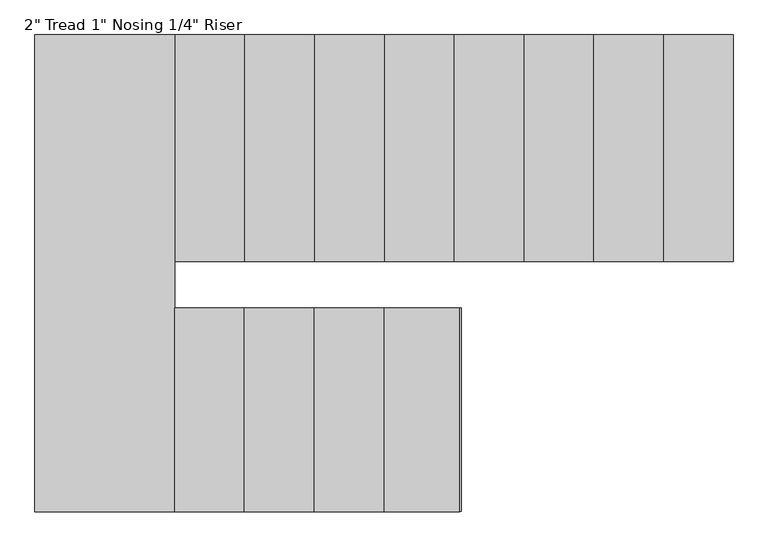
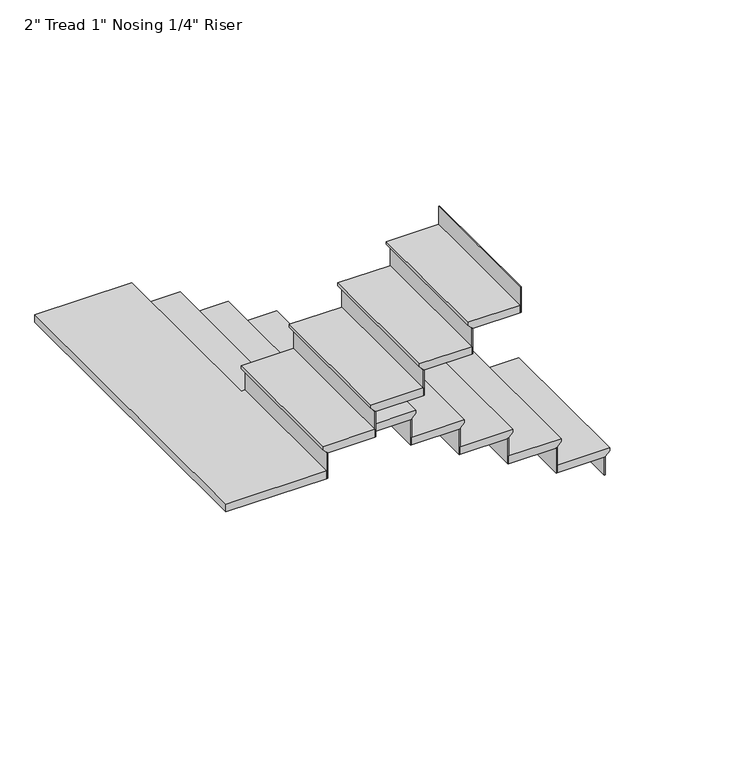
"""IFC4 building model written with IfcOpenShell, lengths in millimetres: stair flight geometry."""

from ifc_helpers import new_model, si_unit, origin, place, context, project, spatial, faceted_brep, source, transform, mapped, element, save


def stair_flight_db34188c(model_context):
    return source(origin(), model_context, "Body", "Brep", [
        faceted_brep([(-569.5630704, 657.3457979, 9599.0833333), (-569.5630704, 657.3457979, 9618.1333333), (-569.5630704, -333.2542021, 9618.1333333), (-569.5630704, -333.2542021, 9599.0833333), (-594.9630704, 657.3457979, 9573.6833333), (-594.9630704, -333.2542021, 9573.6833333), (-899.7630704, 657.3457979, 9618.1333333), (-899.7630704, -333.2542021, 9618.1333333), (-594.9630704, -333.2542021, 9567.3333333), (-899.7630704, -333.2542021, 9567.3333333), (-899.7630704, 657.3457979, 9567.3333333), (-594.9630704, 657.3457979, 9567.3333333)], [[[0, 1, 2, 3]], [[4, 0, 3, 5]], [[2, 1, 6, 7]], [[8, 9, 10, 11]], [[2, 7, 9, 8, 5, 3]], [[8, 11, 4, 5]], [[6, 1, 0, 4, 11, 10]], [[7, 6, 10, 9]]]),
        faceted_brep([(-594.9630704, 657.3457979, 9567.3333333), (-594.9630704, 657.3457979, 9448.8), (-601.3130704, 657.3457979, 9448.8), (-601.3130704, 657.3457979, 9567.3333333), (-594.9630704, -333.2542021, 9567.3333333), (-601.3130704, -333.2542021, 9567.3333333), (-601.3130704, -333.2542021, 9448.8), (-594.9630704, -333.2542021, 9448.8)], [[[0, 1, 2, 3]], [[4, 5, 6, 7]], [[1, 0, 4, 7]], [[2, 1, 7, 6]], [[3, 2, 6, 5]], [[0, 3, 5, 4]]]),
        faceted_brep([(-899.7630704, 657.3457979, 9736.6666667), (-899.7630704, 657.3457979, 9567.3333333), (-906.1130704, 657.3457979, 9567.3333333), (-906.1130704, 657.3457979, 9736.6666667), (-899.7630704, -333.2542021, 9736.6666667), (-906.1130704, -333.2542021, 9736.6666667), (-906.1130704, -333.2542021, 9567.3333333), (-899.7630704, -333.2542021, 9567.3333333)], [[[0, 1, 2, 3]], [[4, 5, 6, 7]], [[1, 0, 4, 7]], [[2, 1, 7, 6]], [[3, 2, 6, 5]], [[0, 3, 5, 4]]]),
        faceted_brep([(-874.3630704, -333.2542021, 9787.4666667), (-874.3630704, 657.3457979, 9787.4666667), (-1204.5630704, 657.3457979, 9787.4666667), (-1204.5630704, -333.2542021, 9787.4666667), (-899.7630704, -333.2542021, 9736.6666667), (-1204.5630704, -333.2542021, 9736.6666667), (-1204.5630704, 657.3457979, 9736.6666667), (-899.7630704, 657.3457979, 9736.6666667), (-899.7630704, -333.2542021, 9743.0166667), (-874.3630704, -333.2542021, 9768.4166667), (-899.7630704, 657.3457979, 9743.0166667), (-874.3630704, 657.3457979, 9768.4166667)], [[[0, 1, 2, 3]], [[4, 5, 6, 7]], [[0, 3, 5, 4, 8, 9]], [[4, 7, 10, 8]], [[2, 1, 11, 10, 7, 6]], [[3, 2, 6, 5]], [[11, 1, 0, 9]], [[10, 11, 9, 8]]]),
        faceted_brep([(-1204.5630704, 657.3457979, 9906.0), (-1204.5630704, 657.3457979, 9736.6666667), (-1210.9130704, 657.3457979, 9736.6666667), (-1210.9130704, 657.3457979, 9906.0), (-1204.5630704, -333.2542021, 9906.0), (-1210.9130704, -333.2542021, 9906.0), (-1210.9130704, -333.2542021, 9736.6666667), (-1204.5630704, -333.2542021, 9736.6666667)], [[[0, 1, 2, 3]], [[4, 5, 6, 7]], [[1, 0, 4, 7]], [[2, 1, 7, 6]], [[3, 2, 6, 5]], [[0, 3, 5, 4]]]),
        faceted_brep([(-1179.1630704, -333.2542021, 9956.8), (-1179.1630704, 657.3457979, 9956.8), (-1509.3630704, 657.3457979, 9956.8), (-1509.3630704, -333.2542021, 9956.8), (-1204.5630704, -333.2542021, 9906.0), (-1509.3630704, -333.2542021, 9906.0), (-1509.3630704, 657.3457979, 9906.0), (-1204.5630704, 657.3457979, 9906.0), (-1204.5630704, -333.2542021, 9912.35), (-1179.1630704, -333.2542021, 9937.75), (-1204.5630704, 657.3457979, 9912.35), (-1179.1630704, 657.3457979, 9937.75)], [[[0, 1, 2, 3]], [[4, 5, 6, 7]], [[0, 3, 5, 4, 8, 9]], [[4, 7, 10, 8]], [[2, 1, 11, 10, 7, 6]], [[3, 2, 6, 5]], [[11, 1, 0, 9]], [[10, 11, 9, 8]]]),
        faceted_brep([(-1509.3630704, 657.3457979, 10075.3333333), (-1509.3630704, 657.3457979, 9906.0), (-1515.7130704, 657.3457979, 9906.0), (-1515.7130704, 657.3457979, 10075.3333333), (-1509.3630704, -333.2542021, 10075.3333333), (-1515.7130704, -333.2542021, 10075.3333333), (-1515.7130704, -333.2542021, 9906.0), (-1509.3630704, -333.2542021, 9906.0)], [[[0, 1, 2, 3]], [[4, 5, 6, 7]], [[1, 0, 4, 7]], [[2, 1, 7, 6]], [[3, 2, 6, 5]], [[0, 3, 5, 4]]]),
        faceted_brep([(-1483.9630704, -333.2542021, 10126.1333333), (-1483.9630704, 657.3457979, 10126.1333333), (-1814.1630704, 657.3457979, 10126.1333333), (-1814.1630704, -333.2542021, 10126.1333333), (-1509.3630704, -333.2542021, 10075.3333333), (-1814.1630704, -333.2542021, 10075.3333333), (-1814.1630704, 657.3457979, 10075.3333333), (-1509.3630704, 657.3457979, 10075.3333333), (-1509.3630704, -333.2542021, 10081.6833333), (-1483.9630704, -333.2542021, 10107.0833333), (-1509.3630704, 657.3457979, 10081.6833333), (-1483.9630704, 657.3457979, 10107.0833333)], [[[0, 1, 2, 3]], [[4, 5, 6, 7]], [[0, 3, 5, 4, 8, 9]], [[4, 7, 10, 8]], [[2, 1, 11, 10, 7, 6]], [[3, 2, 6, 5]], [[11, 1, 0, 9]], [[10, 11, 9, 8]]]),
        faceted_brep([(-1814.1630704, 657.3457979, 10244.6666667), (-1814.1630704, 657.3457979, 10075.3333333), (-1820.5130704, 657.3457979, 10075.3333333), (-1820.5130704, 657.3457979, 10244.6666667), (-1814.1630704, -333.2542021, 10244.6666667), (-1820.5130704, -333.2542021, 10244.6666667), (-1820.5130704, -333.2542021, 10075.3333333), (-1814.1630704, -333.2542021, 10075.3333333)], [[[0, 1, 2, 3]], [[4, 5, 6, 7]], [[1, 0, 4, 7]], [[2, 1, 7, 6]], [[3, 2, 6, 5]], [[0, 3, 5, 4]]]),
        faceted_brep([(-1788.7630704, -333.2542021, 10295.4666667), (-1788.7630704, 657.3457979, 10295.4666667), (-2118.9630704, 657.3457979, 10295.4666667), (-2118.9630704, -333.2542021, 10295.4666667), (-1814.1630704, -333.2542021, 10244.6666667), (-2118.9630704, -333.2542021, 10244.6666667), (-2118.9630704, 657.3457979, 10244.6666667), (-1814.1630704, 657.3457979, 10244.6666667), (-1814.1630704, -333.2542021, 10251.0166667), (-1788.7630704, -333.2542021, 10276.4166667), (-1814.1630704, 657.3457979, 10251.0166667), (-1788.7630704, 657.3457979, 10276.4166667)], [[[0, 1, 2, 3]], [[4, 5, 6, 7]], [[0, 3, 5, 4, 8, 9]], [[4, 7, 10, 8]], [[2, 1, 11, 10, 7, 6]], [[3, 2, 6, 5]], [[11, 1, 0, 9]], [[10, 11, 9, 8]]]),
        faceted_brep([(-2118.9630704, 657.3457979, 10414.0), (-2118.9630704, 657.3457979, 10244.6666667), (-2125.3130704, 657.3457979, 10244.6666667), (-2125.3130704, 657.3457979, 10414.0), (-2118.9630704, -333.2542021, 10414.0), (-2125.3130704, -333.2542021, 10414.0), (-2125.3130704, -333.2542021, 10244.6666667), (-2118.9630704, -333.2542021, 10244.6666667)], [[[0, 1, 2, 3]], [[4, 5, 6, 7]], [[1, 0, 4, 7]], [[2, 1, 7, 6]], [[3, 2, 6, 5]], [[0, 3, 5, 4]]]),
        faceted_brep([(-2093.5630704, -333.2542021, 10464.8), (-2093.5630704, 657.3457979, 10464.8), (-2423.7630704, 657.3457979, 10464.8), (-2423.7630704, -333.2542021, 10464.8), (-2118.9630704, -333.2542021, 10414.0), (-2423.7630704, -333.2542021, 10414.0), (-2423.7630704, 657.3457979, 10414.0), (-2118.9630704, 657.3457979, 10414.0), (-2118.9630704, -333.2542021, 10420.35), (-2093.5630704, -333.2542021, 10445.75), (-2118.9630704, 657.3457979, 10420.35), (-2093.5630704, 657.3457979, 10445.75)], [[[0, 1, 2, 3]], [[4, 5, 6, 7]], [[0, 3, 5, 4, 8, 9]], [[4, 7, 10, 8]], [[2, 1, 11, 10, 7, 6]], [[3, 2, 6, 5]], [[11, 1, 0, 9]], [[10, 11, 9, 8]]]),
        faceted_brep([(-2423.7630704, 657.3457979, 10583.3333333), (-2423.7630704, 657.3457979, 10414.0), (-2430.1130704, 657.3457979, 10414.0), (-2430.1130704, 657.3457979, 10583.3333333), (-2423.7630704, -333.2542021, 10583.3333333), (-2430.1130704, -333.2542021, 10583.3333333), (-2430.1130704, -333.2542021, 10414.0), (-2423.7630704, -333.2542021, 10414.0)], [[[0, 1, 2, 3]], [[4, 5, 6, 7]], [[1, 0, 4, 7]], [[2, 1, 7, 6]], [[3, 2, 6, 5]], [[0, 3, 5, 4]]]),
        faceted_brep([(-2398.3630704, -333.2542021, 10634.1333333), (-2398.3630704, 657.3457979, 10634.1333333), (-2728.5630704, 657.3457979, 10634.1333333), (-2728.5630704, -333.2542021, 10634.1333333), (-2423.7630704, -333.2542021, 10583.3333333), (-2728.5630704, -333.2542021, 10583.3333333), (-2728.5630704, 657.3457979, 10583.3333333), (-2423.7630704, 657.3457979, 10583.3333333), (-2423.7630704, -333.2542021, 10589.6833333), (-2398.3630704, -333.2542021, 10615.0833333), (-2423.7630704, 657.3457979, 10589.6833333), (-2398.3630704, 657.3457979, 10615.0833333)], [[[0, 1, 2, 3]], [[4, 5, 6, 7]], [[0, 3, 5, 4, 8, 9]], [[4, 7, 10, 8]], [[2, 1, 11, 10, 7, 6]], [[3, 2, 6, 5]], [[11, 1, 0, 9]], [[10, 11, 9, 8]]]),
        faceted_brep([(-2728.5630704, 657.3457979, 10752.6666667), (-2728.5630704, 657.3457979, 10583.3333333), (-2734.9130704, 657.3457979, 10583.3333333), (-2734.9130704, 657.3457979, 10752.6666667), (-2728.5630704, -333.2542021, 10752.6666667), (-2734.9130704, -333.2542021, 10752.6666667), (-2734.9130704, -333.2542021, 10583.3333333), (-2728.5630704, -333.2542021, 10583.3333333)], [[[0, 1, 2, 3]], [[4, 5, 6, 7]], [[1, 0, 4, 7]], [[2, 1, 7, 6]], [[3, 2, 6, 5]], [[0, 3, 5, 4]]]),
        faceted_brep([(-2703.1630704, -333.2542021, 10803.4666667), (-2703.1630704, 657.3457979, 10803.4666667), (-3033.3630704, 657.3457979, 10803.4666667), (-3033.3630704, -333.2542021, 10803.4666667), (-2728.5630704, -333.2542021, 10752.6666667), (-3033.3630704, -333.2542021, 10752.6666667), (-3033.3630704, 657.3457979, 10752.6666667), (-2728.5630704, 657.3457979, 10752.6666667), (-2728.5630704, -333.2542021, 10759.0166667), (-2703.1630704, -333.2542021, 10784.4166667), (-2728.5630704, 657.3457979, 10759.0166667), (-2703.1630704, 657.3457979, 10784.4166667)], [[[0, 1, 2, 3]], [[4, 5, 6, 7]], [[0, 3, 5, 4, 8, 9]], [[4, 7, 10, 8]], [[2, 1, 11, 10, 7, 6]], [[3, 2, 6, 5]], [[11, 1, 0, 9]], [[10, 11, 9, 8]]]),
        faceted_brep([(-3033.3630704, 657.3457979, 10922.0), (-3033.3630704, 657.3457979, 10752.6666667), (-3039.7130704, 657.3457979, 10752.6666667), (-3039.7130704, 657.3457979, 10922.0), (-3033.3630704, -333.2542021, 10922.0), (-3039.7130704, -333.2542021, 10922.0), (-3039.7130704, -333.2542021, 10752.6666667), (-3033.3630704, -333.2542021, 10752.6666667)], [[[0, 1, 2, 3]], [[4, 5, 6, 7]], [[1, 0, 4, 7]], [[2, 1, 7, 6]], [[3, 2, 6, 5]], [[0, 3, 5, 4]]]),
        faceted_brep([(-2982.5630704, -536.4542021, 10972.8), (-3007.9630704, -536.4542021, 10972.8), (-3007.9630704, 657.3457979, 10972.8), (-3617.5630704, 657.3457979, 10972.8), (-3617.5630704, -1425.4542021, 10972.8), (-2982.5630704, -1425.4542021, 10972.8), (-3007.9630704, -536.4542021, 10922.0), (-2982.5630704, -536.4542021, 10922.0), (-2982.5630704, -1425.4542021, 10922.0), (-3617.5630704, -1425.4542021, 10922.0), (-3617.5630704, 657.3457979, 10922.0), (-3033.3630704, 657.3457979, 10922.0), (-3033.3630704, -333.2542021, 10922.0), (-3007.9630704, -333.2542021, 10922.0), (-3007.9630704, -333.2542021, 10953.75), (-3007.9630704, 657.3457979, 10953.75), (-3033.3630704, -333.2542021, 10928.35), (-3033.3630704, 657.3457979, 10928.35)], [[[0, 1, 2, 3, 4, 5]], [[6, 7, 8, 9, 10, 11, 12, 13]], [[1, 0, 7, 6]], [[2, 1, 6, 13, 14, 15]], [[13, 12, 16, 14]], [[12, 11, 17, 16]], [[3, 2, 15, 17, 11, 10]], [[4, 3, 10, 9]], [[5, 4, 9, 8]], [[0, 5, 8, 7]], [[17, 15, 14, 16]]]),
        faceted_brep([(-2982.5630704, -1425.4542021, 11091.3333333), (-2982.5630704, -1425.4542021, 10922.0), (-2976.2130704, -1425.4542021, 10922.0), (-2976.2130704, -1425.4542021, 11091.3333333), (-2982.5630704, -536.4542021, 11091.3333333), (-2976.2130704, -536.4542021, 11091.3333333), (-2976.2130704, -536.4542021, 10922.0), (-2982.5630704, -536.4542021, 10922.0)], [[[0, 1, 2, 3]], [[4, 5, 6, 7]], [[1, 0, 4, 7]], [[2, 1, 7, 6]], [[3, 2, 6, 5]], [[0, 3, 5, 4]]]),
        faceted_brep([(-3007.9630704, -536.4542021, 11142.1333333), (-3007.9630704, -1425.4542021, 11142.1333333), (-2677.7630704, -1425.4542021, 11142.1333333), (-2677.7630704, -536.4542021, 11142.1333333), (-2982.5630704, -536.4542021, 11091.3333333), (-2677.7630704, -536.4542021, 11091.3333333), (-2677.7630704, -1425.4542021, 11091.3333333), (-2982.5630704, -1425.4542021, 11091.3333333), (-2982.5630704, -536.4542021, 11097.6833333), (-3007.9630704, -536.4542021, 11123.0833333), (-2982.5630704, -1425.4542021, 11097.6833333), (-3007.9630704, -1425.4542021, 11123.0833333)], [[[0, 1, 2, 3]], [[4, 5, 6, 7]], [[0, 3, 5, 4, 8, 9]], [[4, 7, 10, 8]], [[2, 1, 11, 10, 7, 6]], [[3, 2, 6, 5]], [[11, 1, 0, 9]], [[10, 11, 9, 8]]]),
        faceted_brep([(-2677.7630704, -1425.4542021, 11260.6666667), (-2677.7630704, -1425.4542021, 11091.3333333), (-2671.4130704, -1425.4542021, 11091.3333333), (-2671.4130704, -1425.4542021, 11260.6666667), (-2677.7630704, -536.4542021, 11260.6666667), (-2671.4130704, -536.4542021, 11260.6666667), (-2671.4130704, -536.4542021, 11091.3333333), (-2677.7630704, -536.4542021, 11091.3333333)], [[[0, 1, 2, 3]], [[4, 5, 6, 7]], [[1, 0, 4, 7]], [[2, 1, 7, 6]], [[3, 2, 6, 5]], [[0, 3, 5, 4]]]),
        faceted_brep([(-2703.1630704, -536.4542021, 11311.4666667), (-2703.1630704, -1425.4542021, 11311.4666667), (-2372.9630704, -1425.4542021, 11311.4666667), (-2372.9630704, -536.4542021, 11311.4666667), (-2677.7630704, -536.4542021, 11260.6666667), (-2372.9630704, -536.4542021, 11260.6666667), (-2372.9630704, -1425.4542021, 11260.6666667), (-2677.7630704, -1425.4542021, 11260.6666667), (-2677.7630704, -536.4542021, 11267.0166667), (-2703.1630704, -536.4542021, 11292.4166667), (-2677.7630704, -1425.4542021, 11267.0166667), (-2703.1630704, -1425.4542021, 11292.4166667)], [[[0, 1, 2, 3]], [[4, 5, 6, 7]], [[0, 3, 5, 4, 8, 9]], [[4, 7, 10, 8]], [[2, 1, 11, 10, 7, 6]], [[3, 2, 6, 5]], [[11, 1, 0, 9]], [[10, 11, 9, 8]]]),
        faceted_brep([(-2372.9630704, -1425.4542021, 11430.0), (-2372.9630704, -1425.4542021, 11260.6666667), (-2366.6130704, -1425.4542021, 11260.6666667), (-2366.6130704, -1425.4542021, 11430.0), (-2372.9630704, -536.4542021, 11430.0), (-2366.6130704, -536.4542021, 11430.0), (-2366.6130704, -536.4542021, 11260.6666667), (-2372.9630704, -536.4542021, 11260.6666667)], [[[0, 1, 2, 3]], [[4, 5, 6, 7]], [[1, 0, 4, 7]], [[2, 1, 7, 6]], [[3, 2, 6, 5]], [[0, 3, 5, 4]]]),
        faceted_brep([(-2398.3630704, -536.4542021, 11480.8), (-2398.3630704, -1425.4542021, 11480.8), (-2068.1630704, -1425.4542021, 11480.8), (-2068.1630704, -536.4542021, 11480.8), (-2372.9630704, -536.4542021, 11430.0), (-2068.1630704, -536.4542021, 11430.0), (-2068.1630704, -1425.4542021, 11430.0), (-2372.9630704, -1425.4542021, 11430.0), (-2372.9630704, -536.4542021, 11436.35), (-2398.3630704, -536.4542021, 11461.75), (-2372.9630704, -1425.4542021, 11436.35), (-2398.3630704, -1425.4542021, 11461.75)], [[[0, 1, 2, 3]], [[4, 5, 6, 7]], [[0, 3, 5, 4, 8, 9]], [[4, 7, 10, 8]], [[2, 1, 11, 10, 7, 6]], [[3, 2, 6, 5]], [[11, 1, 0, 9]], [[10, 11, 9, 8]]]),
        faceted_brep([(-2068.1630704, -1425.4542021, 11599.3333333), (-2068.1630704, -1425.4542021, 11430.0), (-2061.8130704, -1425.4542021, 11430.0), (-2061.8130704, -1425.4542021, 11599.3333333), (-2068.1630704, -536.4542021, 11599.3333333), (-2061.8130704, -536.4542021, 11599.3333333), (-2061.8130704, -536.4542021, 11430.0), (-2068.1630704, -536.4542021, 11430.0)], [[[0, 1, 2, 3]], [[4, 5, 6, 7]], [[1, 0, 4, 7]], [[2, 1, 7, 6]], [[3, 2, 6, 5]], [[0, 3, 5, 4]]]),
        faceted_brep([(-1763.3630704, -1425.4542021, 11768.6666667), (-1763.3630704, -1425.4542021, 11599.3333333), (-1757.0130704, -1425.4542021, 11599.3333333), (-1757.0130704, -1425.4542021, 11768.6666667), (-1763.3630704, -536.4542021, 11768.6666667), (-1757.0130704, -536.4542021, 11768.6666667), (-1757.0130704, -536.4542021, 11599.3333333), (-1763.3630704, -536.4542021, 11599.3333333)], [[[0, 1, 2, 3]], [[4, 5, 6, 7]], [[1, 0, 4, 7]], [[2, 1, 7, 6]], [[3, 2, 6, 5]], [[0, 3, 5, 4]]]),
        faceted_brep([(-2093.5630704, -536.4542021, 11650.1333333), (-2093.5630704, -1425.4542021, 11650.1333333), (-1763.3630704, -1425.4542021, 11650.1333333), (-1763.3630704, -536.4542021, 11650.1333333), (-2068.1630704, -536.4542021, 11599.3333333), (-1763.3630704, -536.4542021, 11599.3333333), (-1763.3630704, -1425.4542021, 11599.3333333), (-2068.1630704, -1425.4542021, 11599.3333333), (-2068.1630704, -536.4542021, 11605.6833333), (-2093.5630704, -536.4542021, 11631.0833333), (-2068.1630704, -1425.4542021, 11605.6833333), (-2093.5630704, -1425.4542021, 11631.0833333)], [[[0, 1, 2, 3]], [[4, 5, 6, 7]], [[0, 3, 5, 4, 8, 9]], [[4, 7, 10, 8]], [[2, 1, 11, 10, 7, 6]], [[3, 2, 6, 5]], [[11, 1, 0, 9]], [[10, 11, 9, 8]]]),
    ])


if __name__ == "__main__":
    model = new_model("IFC4")
    model_context = context("Model", 3, world=origin())
    ifc_project = project(units=[si_unit("LENGTHUNIT", "METRE", prefix="MILLI")], contexts=[model_context])
    site = spatial("IfcSite", under=ifc_project)
    building = spatial("IfcBuilding", under=site)
    placement = place(None, origin())
    stair_flight_shape = stair_flight_db34188c(model_context)
    element("IfcStairFlight", 1, ObjectType="2\" Tread 1\" Nosing 1/4\" Riser", at=placement, inside=building, context=model_context, shape_type="MappedRepresentation", body=[
        mapped(stair_flight_shape, transform((0.0, 0.0, 0.0), x_axis=(1.0, 0.0, 0.0), y_axis=(0.0, 1.0, 0.0), z_axis=(0.0, 0.0, 1.0))),
    ])
    save(model, "model.ifc")
